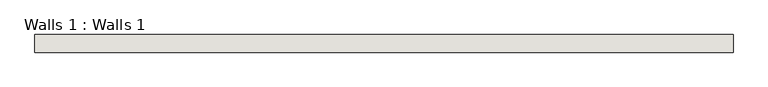
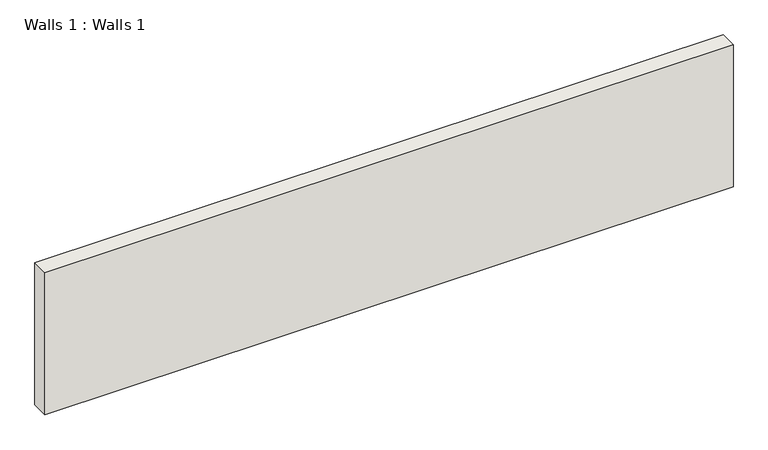
"""IFC4 building model written with IfcOpenShell, lengths in millimetres: wall geometry, Walls 1 : Walls 1."""

from ifc_helpers import new_model, si_unit, origin, origin_with_axes, place, context, project, spatial, polyline, outline, extrude, source, transform, mapped, element, save


def walls_1_walls_1_47b1a65c(model_context):
    return source(origin(), model_context, "Body", "SweptSolid", [
        extrude(outline(polyline([(17863.6339443, -1308.0045164), (5712.2252374, -1308.0045164), (5712.2252374, -1001.0064876), (17863.6339443, -1001.0064876), (17863.6339443, -1308.0045164)])), origin_with_axes(), (0.0, 0.0, 1.0), 2648.0),
    ])


if __name__ == "__main__":
    model = new_model("IFC4")
    model_context = context("Model", 3, world=origin())
    ifc_project = project(units=[si_unit("LENGTHUNIT", "METRE", prefix="MILLI")], contexts=[model_context])
    site = spatial("IfcSite", under=ifc_project)
    building = spatial("IfcBuilding", under=site)
    placement = place(None, origin())
    walls_1_walls_1_shape = walls_1_walls_1_47b1a65c(model_context)
    element("IfcWall", 1, ObjectType="Walls 1 : Walls 1", at=placement, inside=building, context=model_context, shape_type="MappedRepresentation", body=[
        mapped(walls_1_walls_1_shape, transform((0.0, 0.0, 0.0), x_axis=(1.0, 0.0, 0.0), y_axis=(0.0, 1.0, 0.0), z_axis=(0.0, 0.0, 1.0))),
    ])
    save(model, "model.ifc")

# Revit data of these elements
# Element 1 (IfcWall, "Walls 1 : Walls 1")
#   Materials on its faces: "Default Wall"
# Materials
#   "Default Wall": colour RGB 80 80 80, transparency 0
